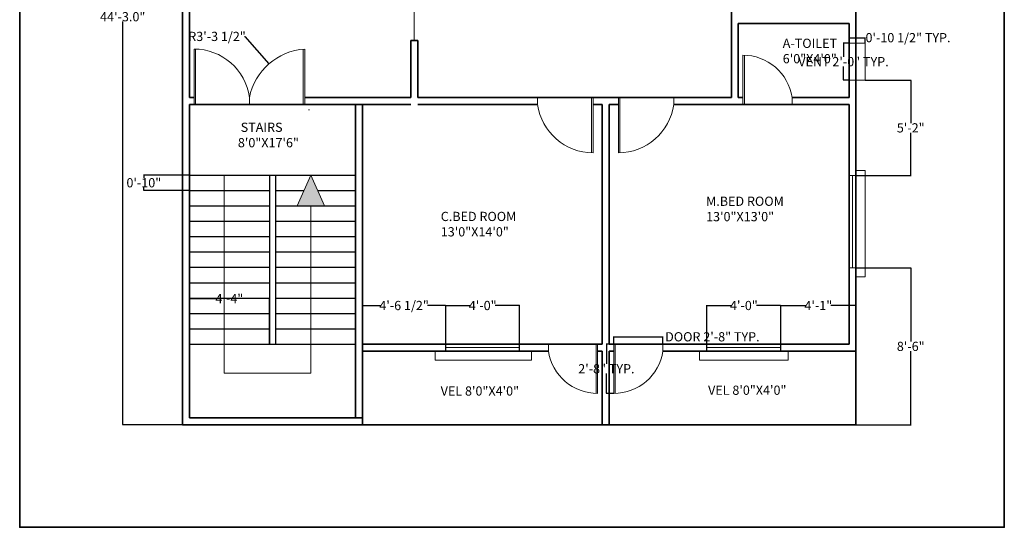
# Model space of a CAD drawing. Units: inches. Extents: x 2946 to 3586, y 7561 to 8235.
# Tile 1 of 2: x 2946 to 3586, y 7561 to 7891. Entities that reach past the tile are written whole.
import ezdxf

# ---------------------------------------------------------------- set-up
doc = ezdxf.new("R2010")
doc.units = ezdxf.units.IN
doc.header["$MEASUREMENT"] = 0
for name, color, linetype, lineweight in [('A-ANNO-DIMS', 2, 'Continuous', 18), ('A-ANNO-PATT', 7, 'Continuous', 18), ('A-ANNO-SYMB', 7, 'Continuous', 18), ('A-ANNO-TTLB', 7, 'Continuous', 35), ('A-AREA-IDEN', 7, 'Continuous', 18), ('A-DOOR', 4, 'Continuous', 18), ('A-FLOR-STRS', 7, 'Continuous', 25), ('A-GLAZ-VENT', 130, 'Continuous', 18), ('A-WALL', 7, 'Continuous', 35), ('windows', 130, 'Continuous', 18)]:
    doc.layers.add(name, color=color, linetype=linetype, lineweight=lineweight)
doc.styles.get("Standard").update_dxf_attribs({"font": 'arial.ttf'})
doc.dimstyles.get("Standard").update_dxf_attribs({"dimtxt": 6, "dimasz": 0.18, "dimexe": 0.18, "dimexo": 0.0625, "dimgap": 0.09, "dimtad": 0, "dimtih": 1, "dimtoh": 1, "dimdec": 1, "dimzin": 0, "dimdsep": 46, "dimlunit": 3, "dimtxsty": 'Standard', "dimcen": 0.09, "dimadec": 0, "dimazin": 0, "dimtfac": 1, "dimtdec": 1, "dimtofl": 0, "dimtmove": 0, "dimatfit": 3, "dimfxl": 1, "dimtolj": 1, "dimtzin": 0, "dimarcsym": 0})

# ---------------------------------------------------------------- blocks, each defined once
blk = doc.blocks.new('*D2')
at = {"layer": 'A-ANNO-DIMS', "color": 0, "lineweight": -2, "transparency": 16777216}
for p, q in [((3051.44, 8158.46), (3012.47, 8158.46)), ((3012.65, 8158.28), (3012.65, 7896.12)), ((3012.65, 7627.64), (3012.65, 7889.81)), ((3051.44, 7627.46), (3012.47, 7627.46))]:
    blk.add_line(p, q, dxfattribs=at)
at = {"layer": 'A-ANNO-DIMS', "color": 0, "transparency": 16777216}
for points in [[(3012.62, 8158.28), (3012.68, 8158.28), (3012.65, 8158.46)], [(3012.62, 7627.64), (3012.68, 7627.64), (3012.65, 7627.46)]]:
    blk.add_solid(points, dxfattribs=at)
at = {"layer": 'Defpoints', "color": 0, "transparency": 16777216}
for p in [(3051.51, 8158.46), (3012.65, 7627.46), (3051.51, 7627.46)]:
    blk.add_point(p, dxfattribs=at)
at = {"layer": 'A-ANNO-DIMS', "color": 0, "transparency": 16777216, "insert": (3012.65, 7892.96), "char_height": 6, "attachment_point": 5}
blk.add_mtext('\\A1;44\'-3.0"', dxfattribs=at)
blk = doc.blocks.new('DOOR-SINGLE-36IN')
for p, q in [((-1, 36), (-1, 0)), ((0, 0), (0, 36)), ((0, 36), (0, 0)), ((-36, 0), (-36, 4.5)), ((0, 0), (-36, 0))]:
    blk.add_line(p, q)
blk.add_arc((0, -0.32), 36.32, 90, 172.37185)
blk = doc.blocks.new('DOOR-SINGLE-32IN')
for p, q in [((0, 0), (0, -32)), ((0, -32), (0, 0)), ((0, 0), (32, 0)), ((1, -32), (1, 0)), ((32, 0), (32, -4.5))]:
    blk.add_line(p, q)
blk.add_arc((0, 0.37), 32.37, 270, 351.34988)
blk = doc.blocks.new('WIN-60IN')
for p, q in [((0, 0), (0, -4.5)), ((60, 0), (0, 0)), ((0, -2.25), (60, -2.25)), ((0, -4.5), (60, -4.5)), ((60, -4.5), (60, 0))]:
    blk.add_line(p, q)
blk = doc.blocks.new('WIN-SILL-60IN')
for p, q in [((0, 0), (0, 6)), ((0, 6), (69.18, 6)), ((69.18, 6), (69.18, 0))]:
    blk.add_line(p, q)
blk = doc.blocks.new('VENT-24IN')
for p, q in [((0, 0), (4.5, 0)), ((0, -24), (0, 0)), ((4.5, 0), (4.5, -24)), ((4.5, 0), (10.5, 0)), ((10.5, 0), (10.5, -24)), ((4.5, -24), (0, -24)), ((10.5, -24), (4.5, -24))]:
    blk.add_line(p, q)
blk = doc.blocks.new('*D14')
at = {"layer": 'A-ANNO-DIMS', "color": 0, "lineweight": -2, "transparency": 16777216}
for p, q in [((3332.01, 7680.02), (3332.01, 7684.94)), ((3332.19, 7684.76), (3363.83, 7684.76)), ((3364.01, 7680.02), (3364.01, 7684.94)), ((3364.01, 7684.76), (3364.19, 7684.76))]:
    blk.add_line(p, q, dxfattribs=at)
at = {"layer": 'A-ANNO-DIMS', "color": 0, "transparency": 16777216}
for points in [[(3332.19, 7684.79), (3332.19, 7684.73), (3332.01, 7684.76)], [(3363.83, 7684.79), (3363.83, 7684.73), (3364.01, 7684.76)]]:
    blk.add_solid(points, dxfattribs=at)
at = {"layer": 'Defpoints', "color": 0, "transparency": 16777216}
for p in [(3364.01, 7684.76), (3332.01, 7679.96), (3364.01, 7679.96)]:
    blk.add_point(p, dxfattribs=at)
at = {"layer": 'A-ANNO-DIMS', "color": 0, "transparency": 16777216, "insert": (3396.15, 7684.76), "char_height": 6, "attachment_point": 5}
blk.add_mtext('\\A1;DOOR 2\'-8" TYP.', dxfattribs=at)
blk = doc.blocks.new('*D15')
at = {"layer": 'A-ANNO-DIMS', "color": 0, "lineweight": -2, "transparency": 16777216}
for p, q in [((3331.94, 7679.96), (3327.03, 7679.96)), ((3327.21, 7679.78), (3327.21, 7667.12)), ((3327.21, 7648.14), (3327.21, 7660.81)), ((3331.94, 7647.96), (3327.03, 7647.96))]:
    blk.add_line(p, q, dxfattribs=at)
at = {"layer": 'A-ANNO-DIMS', "color": 0, "transparency": 16777216}
for points in [[(3327.18, 7679.78), (3327.24, 7679.78), (3327.21, 7679.96)], [(3327.18, 7648.14), (3327.24, 7648.14), (3327.21, 7647.96)]]:
    blk.add_solid(points, dxfattribs=at)
at = {"layer": 'Defpoints', "color": 0, "transparency": 16777216}
for p in [(3327.21, 7679.96), (3332.01, 7679.96), (3332.01, 7647.96)]:
    blk.add_point(p, dxfattribs=at)
at = {"layer": 'A-ANNO-DIMS', "color": 0, "transparency": 16777216, "insert": (3327.21, 7663.96), "char_height": 6, "attachment_point": 5}
blk.add_mtext('\\A1;2\'-8" TYP.', dxfattribs=at)
blk = doc.blocks.new('*D16')
at = {"layer": 'A-ANNO-DIMS', "color": 0, "lineweight": -2, "transparency": 16777216}
for p, q in [((3484.94, 7875.73), (3481.23, 7875.73)), ((3481.41, 7875.55), (3481.41, 7866.89)), ((3481.41, 7851.91), (3481.41, 7860.58)), ((3484.94, 7851.73), (3481.23, 7851.73))]:
    blk.add_line(p, q, dxfattribs=at)
at = {"layer": 'A-ANNO-DIMS', "color": 0, "transparency": 16777216}
for points in [[(3481.38, 7875.55), (3481.44, 7875.55), (3481.41, 7875.73)], [(3481.38, 7851.91), (3481.44, 7851.91), (3481.41, 7851.73)]]:
    blk.add_solid(points, dxfattribs=at)
at = {"layer": 'Defpoints', "color": 0, "transparency": 16777216}
for p in [(3481.41, 7875.73), (3485.01, 7875.73), (3485.01, 7851.73)]:
    blk.add_point(p, dxfattribs=at)
at = {"layer": 'A-ANNO-DIMS', "color": 0, "transparency": 16777216, "insert": (3481.41, 7863.73), "char_height": 6, "attachment_point": 5}
blk.add_mtext('\\A1;VENT 2\'-0" TYP.', dxfattribs=at)
blk = doc.blocks.new('*D17')
at = {"layer": 'A-ANNO-DIMS', "color": 0, "lineweight": -2, "transparency": 16777216}
for p, q in [((3485.01, 7875.79), (3485.01, 7879.51)), ((3485.19, 7879.33), (3495.33, 7879.33)), ((3495.51, 7875.79), (3495.51, 7879.51)), ((3495.51, 7879.33), (3495.69, 7879.33))]:
    blk.add_line(p, q, dxfattribs=at)
at = {"layer": 'A-ANNO-DIMS', "color": 0, "transparency": 16777216}
for points in [[(3485.19, 7879.36), (3485.19, 7879.3), (3485.01, 7879.33)], [(3495.33, 7879.36), (3495.33, 7879.3), (3495.51, 7879.33)]]:
    blk.add_solid(points, dxfattribs=at)
at = {"layer": 'Defpoints', "color": 0, "transparency": 16777216}
for p in [(3495.51, 7879.33), (3485.01, 7875.73), (3495.51, 7875.73)]:
    blk.add_point(p, dxfattribs=at)
at = {"layer": 'A-ANNO-DIMS', "color": 0, "transparency": 16777216, "insert": (3523.39, 7879.33), "char_height": 6, "attachment_point": 5}
blk.add_mtext('\\A1;0\'-10 1/2" TYP.', dxfattribs=at)
blk = doc.blocks.new('*D26')
at = {"layer": 'A-ANNO-DIMS', "color": 0, "lineweight": -2, "transparency": 16777216}
for p, q in [((3495.57, 7851.73), (3525.34, 7851.73)), ((3525.16, 7851.55), (3525.16, 7823.82)), ((3525.16, 7789.79), (3525.16, 7817.52)), ((3489.57, 7789.61), (3525.34, 7789.61))]:
    blk.add_line(p, q, dxfattribs=at)
at = {"layer": 'A-ANNO-DIMS', "color": 0, "transparency": 16777216}
for points in [[(3525.13, 7851.55), (3525.19, 7851.55), (3525.16, 7851.73)], [(3525.13, 7789.79), (3525.19, 7789.79), (3525.16, 7789.61)]]:
    blk.add_solid(points, dxfattribs=at)
at = {"layer": 'Defpoints', "color": 0, "transparency": 16777216}
for p in [(3495.51, 7851.73), (3525.16, 7851.73), (3489.51, 7789.61)]:
    blk.add_point(p, dxfattribs=at)
at = {"layer": 'A-ANNO-DIMS', "color": 0, "transparency": 16777216, "insert": (3525.16, 7820.67), "char_height": 6, "attachment_point": 5}
blk.add_mtext('\\A1;5\'-2"', dxfattribs=at)
blk = doc.blocks.new('*D27')
at = {"layer": 'A-ANNO-DIMS', "color": 0, "lineweight": -2, "transparency": 16777216}
for p, q in [((3489.57, 7729.61), (3525.34, 7729.61)), ((3525.16, 7729.43), (3525.16, 7681.69)), ((3525.16, 7627.64), (3525.16, 7675.38)), ((3489.57, 7627.46), (3525.34, 7627.46))]:
    blk.add_line(p, q, dxfattribs=at)
at = {"layer": 'A-ANNO-DIMS', "color": 0, "transparency": 16777216}
for points in [[(3525.13, 7729.43), (3525.19, 7729.43), (3525.16, 7729.61)], [(3525.13, 7627.64), (3525.19, 7627.64), (3525.16, 7627.46)]]:
    blk.add_solid(points, dxfattribs=at)
at = {"layer": 'Defpoints', "color": 0, "transparency": 16777216}
for p in [(3489.51, 7729.61), (3525.16, 7729.61), (3489.51, 7627.46)]:
    blk.add_point(p, dxfattribs=at)
at = {"layer": 'A-ANNO-DIMS', "color": 0, "transparency": 16777216, "insert": (3525.16, 7678.53), "char_height": 6, "attachment_point": 5}
blk.add_mtext('\\A1;8\'-6"', dxfattribs=at)
blk = doc.blocks.new('*D28')
at = {"layer": 'A-ANNO-DIMS', "color": 0, "lineweight": -2, "transparency": 16777216}
for p, q in [((3056.01, 7680.02), (3056.01, 7709.79)), ((3056.19, 7709.61), (3073.82, 7709.61)), ((3107.83, 7709.61), (3090.19, 7709.61)), ((3108.01, 7680.02), (3108.01, 7709.79))]:
    blk.add_line(p, q, dxfattribs=at)
at = {"layer": 'A-ANNO-DIMS', "color": 0, "transparency": 16777216}
for points in [[(3056.19, 7709.64), (3056.19, 7709.58), (3056.01, 7709.61)], [(3107.83, 7709.64), (3107.83, 7709.58), (3108.01, 7709.61)]]:
    blk.add_solid(points, dxfattribs=at)
at = {"layer": 'Defpoints', "color": 0, "transparency": 16777216}
for p in [(3108.01, 7709.61), (3056.01, 7679.96), (3108.01, 7679.96)]:
    blk.add_point(p, dxfattribs=at)
at = {"layer": 'A-ANNO-DIMS', "color": 0, "transparency": 16777216, "insert": (3082.01, 7709.61), "char_height": 6, "attachment_point": 5}
blk.add_mtext('\\A1;4\'-4"', dxfattribs=at)
blk = doc.blocks.new('*D29')
at = {"layer": 'A-ANNO-DIMS', "color": 0, "lineweight": -2, "transparency": 16777216}
for p, q in [((3055.94, 7789.96), (3026.18, 7789.96)), ((3026.36, 7789.78), (3026.36, 7788.12)), ((3026.36, 7780.14), (3026.36, 7781.81)), ((3055.94, 7779.96), (3026.18, 7779.96))]:
    blk.add_line(p, q, dxfattribs=at)
at = {"layer": 'A-ANNO-DIMS', "color": 0, "transparency": 16777216}
for points in [[(3026.33, 7789.78), (3026.39, 7789.78), (3026.36, 7789.96)], [(3026.33, 7780.14), (3026.39, 7780.14), (3026.36, 7779.96)]]:
    blk.add_solid(points, dxfattribs=at)
at = {"layer": 'Defpoints', "color": 0, "transparency": 16777216}
for p in [(3026.36, 7789.96), (3056.01, 7789.96), (3056.01, 7779.96)]:
    blk.add_point(p, dxfattribs=at)
at = {"layer": 'A-ANNO-DIMS', "color": 0, "transparency": 16777216, "insert": (3026.36, 7784.96), "char_height": 6, "attachment_point": 5}
blk.add_mtext('\\A1;0\'-10"', dxfattribs=at)
blk = doc.blocks.new('*D30')
at = {"layer": 'A-ANNO-DIMS', "color": 0, "lineweight": -2, "transparency": 16777216}
for p, q in [((3168.51, 7675.52), (3168.51, 7705.29)), ((3168.69, 7705.11), (3180.47, 7705.11)), ((3222.6, 7705.11), (3210.82, 7705.11)), ((3222.78, 7675.52), (3222.78, 7705.29))]:
    blk.add_line(p, q, dxfattribs=at)
at = {"layer": 'A-ANNO-DIMS', "color": 0, "transparency": 16777216}
for points in [[(3168.69, 7705.14), (3168.69, 7705.08), (3168.51, 7705.11)], [(3222.6, 7705.14), (3222.6, 7705.08), (3222.78, 7705.11)]]:
    blk.add_solid(points, dxfattribs=at)
at = {"layer": 'Defpoints', "color": 0, "transparency": 16777216}
for p in [(3222.78, 7705.11), (3168.51, 7675.46), (3222.78, 7675.46)]:
    blk.add_point(p, dxfattribs=at)
at = {"layer": 'A-ANNO-DIMS', "color": 0, "transparency": 16777216, "insert": (3195.64, 7705.11), "char_height": 6, "attachment_point": 5}
blk.add_mtext('\\A1;4\'-6 1/2"', dxfattribs=at)
blk = doc.blocks.new('*D31')
at = {"layer": 'A-ANNO-DIMS', "color": 0, "lineweight": -2, "transparency": 16777216}
for p, q in [((3222.78, 7675.52), (3222.78, 7705.29)), ((3222.96, 7705.11), (3238.59, 7705.11)), ((3270.6, 7705.11), (3254.97, 7705.11)), ((3270.78, 7675.52), (3270.78, 7705.29))]:
    blk.add_line(p, q, dxfattribs=at)
at = {"layer": 'A-ANNO-DIMS', "color": 0, "transparency": 16777216}
for points in [[(3222.96, 7705.14), (3222.96, 7705.08), (3222.78, 7705.11)], [(3270.6, 7705.14), (3270.6, 7705.08), (3270.78, 7705.11)]]:
    blk.add_solid(points, dxfattribs=at)
at = {"layer": 'Defpoints', "color": 0, "transparency": 16777216}
for p in [(3270.78, 7705.11), (3222.78, 7675.46), (3270.78, 7675.46)]:
    blk.add_point(p, dxfattribs=at)
at = {"layer": 'A-ANNO-DIMS', "color": 0, "transparency": 16777216, "insert": (3246.78, 7705.11), "char_height": 6, "attachment_point": 5}
blk.add_mtext('\\A1;4\'-0"', dxfattribs=at)
blk = doc.blocks.new('*D32')
at = {"layer": 'A-ANNO-DIMS', "color": 0, "lineweight": -2, "transparency": 16777216}
for p, q in [((3392.63, 7675.52), (3392.63, 7705.29)), ((3392.81, 7705.11), (3408.45, 7705.11)), ((3440.45, 7705.11), (3424.82, 7705.11)), ((3440.63, 7675.52), (3440.63, 7705.29))]:
    blk.add_line(p, q, dxfattribs=at)
at = {"layer": 'A-ANNO-DIMS', "color": 0, "transparency": 16777216}
for points in [[(3392.81, 7705.14), (3392.81, 7705.08), (3392.63, 7705.11)], [(3440.45, 7705.14), (3440.45, 7705.08), (3440.63, 7705.11)]]:
    blk.add_solid(points, dxfattribs=at)
at = {"layer": 'Defpoints', "color": 0, "transparency": 16777216}
for p in [(3440.63, 7705.11), (3392.63, 7675.46), (3440.63, 7675.46)]:
    blk.add_point(p, dxfattribs=at)
at = {"layer": 'A-ANNO-DIMS', "color": 0, "transparency": 16777216, "insert": (3416.63, 7705.11), "char_height": 6, "attachment_point": 5}
blk.add_mtext('\\A1;4\'-0"', dxfattribs=at)
blk = doc.blocks.new('*D33')
at = {"layer": 'A-ANNO-DIMS', "color": 0, "lineweight": -2, "transparency": 16777216}
for p, q in [((3440.63, 7675.52), (3440.63, 7705.29)), ((3440.81, 7705.11), (3456.88, 7705.11)), ((3489.33, 7705.11), (3473.26, 7705.11)), ((3489.51, 7675.52), (3489.51, 7705.29))]:
    blk.add_line(p, q, dxfattribs=at)
at = {"layer": 'A-ANNO-DIMS', "color": 0, "transparency": 16777216}
for points in [[(3440.81, 7705.14), (3440.81, 7705.08), (3440.63, 7705.11)], [(3489.33, 7705.14), (3489.33, 7705.08), (3489.51, 7705.11)]]:
    blk.add_solid(points, dxfattribs=at)
at = {"layer": 'Defpoints', "color": 0, "transparency": 16777216}
for p in [(3489.51, 7705.11), (3440.63, 7675.46), (3489.51, 7675.46)]:
    blk.add_point(p, dxfattribs=at)
at = {"layer": 'A-ANNO-DIMS', "color": 0, "transparency": 16777216, "insert": (3465.07, 7705.11), "char_height": 6, "attachment_point": 5}
blk.add_mtext('\\A1;4\'-1"', dxfattribs=at)
blk = doc.blocks.new('*D34')
at = {"layer": 'A-ANNO-DIMS', "color": 0, "lineweight": -2, "transparency": 16777216}
for p, q in [((3091.88, 7880.15), (3092.06, 7880.15)), ((3092.06, 7880.15), (3107.6, 7862.39)), ((3133.71, 7832.44), (3133.89, 7832.44)), ((3133.8, 7832.35), (3133.8, 7832.53))]:
    blk.add_line(p, q, dxfattribs=at)
at = {"layer": 'A-ANNO-DIMS', "color": 0, "transparency": 16777216}
blk.add_solid([(3107.62, 7862.41), (3107.58, 7862.37), (3107.72, 7862.26)], dxfattribs=at)
at = {"layer": 'Defpoints', "color": 0, "transparency": 16777216}
for p in [(3107.72, 7862.26), (3133.8, 7832.44)]:
    blk.add_point(p, dxfattribs=at)
at = {"layer": 'A-ANNO-DIMS', "color": 0, "transparency": 16777216, "insert": (3073.96, 7880.15), "char_height": 6, "attachment_point": 5}
blk.add_mtext('\\A1;R3\'-3 1/2"', dxfattribs=at)

msp = doc.modelspace()

# ---------------------------------------------------------------- hatches: boundary and pattern name
at = {"layer": 'A-ANNO-PATT'}
h = msp.add_hatch(color=256, dxfattribs=at)
h.dxf.hatch_style = 1
h.paths.add_polyline_path([(3134.98, 7789.96), (3126.01, 7769.96), (3143.96, 7769.96)])

# ---------------------------------------------------------------- linework, layer by layer
at = {"layer": 'A-ANNO-SYMB'}
for p, q in [((3078.69, 7789.96), (3078.69, 7661.05)), ((3134.98, 7789.96), (3126.01, 7769.96)), ((3134.98, 7789.96), (3143.96, 7769.96)), ((3126.01, 7769.96), (3143.96, 7769.96)), ((3134.98, 7661.05), (3134.98, 7769.96)), ((3078.69, 7661.05), (3134.98, 7661.05))]:
    msp.add_line(p, q, dxfattribs=at)
at = {"layer": 'A-ANNO-TTLB'}
msp.add_lwpolyline([(2945.62, 8234.75), (3586.02, 8234.75), (3586.02, 7560.83), (2945.62, 7560.83)], close=True, dxfattribs=at)
at = {"layer": 'A-DOOR'}
for p, q in [((3059.01, 7835.96), (3059.01, 7871.96)), ((3059.01, 7871.96), (3059.01, 7835.96)), ((3060.01, 7871.96), (3060.01, 7835.96)), ((3130.01, 7871.96), (3130.01, 7835.96)), ((3131.01, 7835.96), (3131.01, 7871.96)), ((3131.01, 7871.96), (3131.01, 7835.96)), ((3095.01, 7835.96), (3095.01, 7840.46)), ((3095.01, 7840.46), (3095.01, 7835.96)), ((3059.01, 7835.96), (3095.01, 7835.96)), ((3095.01, 7835.96), (3131.01, 7835.96))]:
    msp.add_line(p, q, dxfattribs=at)
for centre, radius, start, end in [((3059.01, 7835.64), 36.32, 7.62815, 90), ((3133.8, 7832.44), 39.62, 94.04721, 168.32464)]:
    msp.add_arc(centre, radius, start, end, dxfattribs=at)
at = {"layer": 'A-FLOR-STRS'}
for p, q in [((3056.01, 7789.96), (3164.01, 7789.96)), ((3108.01, 7789.96), (3108.01, 7679.96)), ((3112.01, 7789.96), (3112.01, 7679.96)), ((3056.01, 7779.96), (3108.01, 7779.96)), ((3056.01, 7779.96), (3108.01, 7779.96)), ((3112.01, 7779.96), (3130.49, 7779.96)), ((3112.01, 7779.96), (3126.01, 7779.96)), ((3139.47, 7779.96), (3164.01, 7779.96)), ((3056.01, 7769.96), (3108.01, 7769.96)), ((3056.01, 7769.96), (3108.01, 7769.96)), ((3112.01, 7769.96), (3126.01, 7769.96)), ((3112.01, 7769.96), (3164.01, 7769.96)), ((3056.01, 7759.96), (3108.01, 7759.96)), ((3056.01, 7759.96), (3108.01, 7759.96)), ((3112.01, 7759.96), (3126.01, 7759.96)), ((3112.01, 7759.96), (3164.01, 7759.96)), ((3056.01, 7749.96), (3108.01, 7749.96)), ((3056.01, 7749.96), (3108.01, 7749.96)), ((3112.01, 7749.96), (3126.01, 7749.96)), ((3112.01, 7749.96), (3164.01, 7749.96)), ((3056.01, 7739.96), (3108.01, 7739.96)), ((3056.01, 7739.96), (3108.01, 7739.96)), ((3112.01, 7739.96), (3126.01, 7739.96)), ((3112.01, 7739.96), (3164.01, 7739.96)), ((3056.01, 7729.96), (3108.01, 7729.96)), ((3056.01, 7729.96), (3108.01, 7729.96)), ((3112.01, 7729.96), (3164.01, 7729.96)), ((3112.01, 7729.96), (3126.01, 7729.96)), ((3056.01, 7719.96), (3108.01, 7719.96)), ((3056.01, 7719.96), (3108.01, 7719.96)), ((3112.01, 7719.96), (3164.01, 7719.96)), ((3112.01, 7719.96), (3126.01, 7719.96)), ((3056.01, 7709.96), (3108.01, 7709.96)), ((3056.01, 7709.96), (3108.01, 7709.96)), ((3112.01, 7709.96), (3126.01, 7709.96)), ((3112.01, 7709.96), (3164.01, 7709.96)), ((3056.01, 7699.96), (3108.01, 7699.96)), ((3056.01, 7699.96), (3108.01, 7699.96)), ((3112.01, 7699.96), (3126.01, 7699.96)), ((3112.01, 7699.96), (3164.01, 7699.96)), ((3056.01, 7689.96), (3108.01, 7689.96)), ((3056.01, 7689.96), (3108.01, 7689.96)), ((3112.01, 7689.96), (3126.01, 7689.96)), ((3112.01, 7689.96), (3164.01, 7689.96)), ((3056.01, 7679.96), (3164.01, 7679.96))]:
    msp.add_line(p, q, dxfattribs=at)
at = {"layer": 'A-WALL'}
for p, q in [((3051.51, 8158.46), (3051.51, 7627.46)), ((3489.51, 8158.46), (3489.51, 7627.46)), ((3056.01, 7993.46), (3056.01, 7840.46)), ((3408.51, 7993.46), (3408.51, 7840.46)), ((3413.01, 7888.46), (3485.01, 7888.46)), ((3413.01, 7888.46), (3413.01, 7840.46)), ((3485.01, 7888.46), (3485.01, 7840.46)), ((3200.01, 7877.43), (3204.51, 7877.43)), ((3200.01, 7877.43), (3200.01, 7840.46)), ((3204.51, 7877.43), (3204.51, 7840.46)), ((3056.01, 7840.46), (3059.01, 7840.46)), ((3131.01, 7840.46), (3200.01, 7840.46)), ((3204.51, 7840.46), (3408.51, 7840.46)), ((3324.51, 7840.46), (3318.51, 7840.46)), ((3329.01, 7840.46), (3335.01, 7840.46)), ((3413.01, 7840.46), (3416.01, 7840.46)), ((3448.01, 7840.46), (3485.01, 7840.46)), ((3056.01, 7835.96), (3200.01, 7835.96)), ((3056.01, 7835.96), (3059.01, 7835.96)), ((3056.01, 7835.96), (3056.01, 7631.96)), ((3164.01, 7835.96), (3164.01, 7679.96)), ((3168.51, 7835.96), (3168.51, 7679.96)), ((3204.51, 7835.96), (3282.51, 7835.96)), ((3318.51, 7835.96), (3324.51, 7835.96)), ((3324.51, 7835.96), (3324.51, 7679.96)), ((3329.01, 7835.96), (3329.01, 7679.96)), ((3329.01, 7835.96), (3335.01, 7835.96)), ((3371.01, 7835.96), (3485.01, 7835.96)), ((3413.01, 7835.96), (3416.01, 7835.96)), ((3485.01, 7835.96), (3485.01, 7679.96)), ((3164.01, 7679.96), (3164.01, 7631.96)), ((3168.51, 7679.96), (3168.51, 7627.46)), ((3168.51, 7679.96), (3200.01, 7679.96)), ((3200.01, 7679.96), (3324.51, 7679.96)), ((3324.51, 7679.96), (3321.51, 7679.96)), ((3329.01, 7679.96), (3332.01, 7679.96)), ((3329.01, 7679.96), (3485.01, 7679.96)), ((3056.01, 7631.96), (3056.01, 7675.46)), ((3168.51, 7675.46), (3200.01, 7675.46)), ((3200.01, 7675.46), (3289.51, 7675.46)), ((3321.51, 7675.46), (3324.51, 7675.46)), ((3324.51, 7675.46), (3324.51, 7627.46)), ((3329.01, 7675.46), (3329.01, 7627.46)), ((3329.01, 7675.46), (3332.01, 7675.46)), ((3364.01, 7675.46), (3489.51, 7675.46)), ((3051.51, 7631.96), (3051.51, 7631.96)), ((3051.51, 7627.46), (3489.51, 7627.46)), ((3056.01, 7631.96), (3168.51, 7631.96))]:
    msp.add_line(p, q, dxfattribs=at)
at = {"layer": 'windows'}
for p, q in [((3202.26, 7965.14), (3202.26, 7877.43)), ((3222.78, 7679.96), (3222.78, 7675.46)), ((3270.51, 7679.96), (3222.78, 7679.96)), ((3270.78, 7675.46), (3270.51, 7679.96)), ((3392.63, 7675.46), (3392.63, 7679.96)), ((3392.63, 7679.96), (3440.63, 7679.96)), ((3440.63, 7679.96), (3440.63, 7675.46)), ((3215.94, 7669.46), (3215.94, 7675.46)), ((3222.78, 7677.71), (3270.64, 7677.71)), ((3222.78, 7675.46), (3222.78, 7675.46)), ((3222.78, 7675.46), (3270.78, 7675.46)), ((3278.49, 7675.46), (3278.49, 7669.46)), ((3387.86, 7669.46), (3387.86, 7675.46)), ((3392.63, 7677.71), (3440.63, 7677.71)), ((3440.63, 7675.46), (3392.63, 7675.46)), ((3445.4, 7675.46), (3445.4, 7669.46)), ((3278.49, 7669.46), (3215.94, 7669.46)), ((3445.4, 7669.46), (3387.86, 7669.46))]:
    msp.add_line(p, q, dxfattribs=at)

# ---------------------------------------------------------------- block references
at = {"layer": 'A-DOOR', "extrusion": (0, 0, -1), "zscale": -1, "rotation": 180}
for name, p in [('DOOR-SINGLE-32IN', (-3416.01, 7835.96)), ('DOOR-SINGLE-36IN', (-3318.51, 7840.46))]:
    msp.add_blockref(name, p, dxfattribs=at)
at = {"layer": 'A-DOOR', "rotation": 180}
msp.add_blockref('DOOR-SINGLE-36IN', (3335.01, 7840.46), dxfattribs=at)
at = {"layer": 'A-DOOR', "extrusion": (0, 0, -1), "zscale": -1}
msp.add_blockref('DOOR-SINGLE-32IN', (-3321.51, 7679.96), dxfattribs=at)
at = {"layer": 'A-DOOR'}
msp.add_blockref('DOOR-SINGLE-32IN', (3332.01, 7679.96), dxfattribs=at)
at = {"layer": 'A-GLAZ-VENT'}
msp.add_blockref('VENT-24IN', (3485.01, 7875.73), dxfattribs=at)
at = {"layer": 'windows'}
for name, p, rotation in [('WIN-60IN', (3485.01, 7729.61), 90.00000000000202), ('WIN-SILL-60IN', (3489.51, 7793.02), 269.9999999999998)]:
    msp.add_blockref(name, p, dxfattribs=dict(at, rotation=rotation))

# ---------------------------------------------------------------- texts
at = {"layer": 'A-AREA-IDEN', "char_height": 6, "attachment_point": 1}
for s, width, insert in [('A-TOILET\\P6\'0"X4\'0"', 38.2975, (3441.9, 7878.67)), (' STAIRS\\P8\'0"X17\'6"', 71.4212, (3087.53, 7824.04)), ('M.BED ROOM\\P13\'0"X13\'0"', 98.5773, (3392.04, 7775.94)), ('C.BED ROOM\\P13\'0"X14\'0"', 107.1422, (3219.49, 7766.05)), ('VEL 8\'0"X4\'0"', 99.933, (3219.44, 7652.5)), ('VEL 8\'0"X4\'0"', 99.933, (3393.35, 7653.01)), ('VEL 8\'0"X4\'0"', 99.933, (3393.35, 7653.01))]:
    msp.add_mtext_dynamic_manual_height_columns(s, width=width, gutter_width=1, heights=[0], dxfattribs=dict(at, insert=insert))

# ---------------------------------------------------------------- dimensions: what is measured, and where the dimension line sits
at = {"layer": 'A-ANNO-DIMS'}
for base, p1, p2, override, picture, middle in [((3012.65, 7627.46), (3051.51, 8158.46), (3051.51, 7627.46), {"dimclrd": 0, "dimclre": 0, "dimclrt": 0}, '*D2', (3012.65, 7892.96)), ((3525.16, 7851.73), (3489.51, 7789.61), (3495.51, 7851.73), {"dimdec": 1, "dimlfac": 1, "dimrnd": 0, "dimzin": 1, "dimdsep": 46, "dimlunit": 4, "dimfrac": 2}, '*D26', (3525.16, 7820.67)), ((3026.36, 7789.96), (3056.01, 7779.96), (3056.01, 7789.96), {"dimdec": 1, "dimlfac": 1, "dimrnd": 0, "dimzin": 1, "dimdsep": 46, "dimlunit": 4, "dimfrac": 2}, '*D29', (3026.36, 7784.96)), ((3525.1574, 7729.6073), (3489.5074, 7627.4616), (3489.5074, 7729.6073), {"dimdec": 1, "dimlfac": 1, "dimrnd": 0, "dimzin": 1, "dimdsep": 46, "dimlunit": 4, "dimfrac": 2}, '*D27', (3525.1574, 7678.5344))]:
    dim = msp.add_linear_dim(base=base, p1=p1, p2=p2, angle=90, dimstyle='Standard', override=override, dxfattribs=at)
    dim.commit()
    dim.dimension.update_dxf_attribs({"geometry": picture, "text_midpoint": middle})
for base, p1, p2, text, picture, middle in [((3495.51, 7879.33), (3485.01, 7875.73), (3495.51, 7875.73), '<> TYP.', '*D17', (3523.39, 7879.33)), ((3364.01, 7684.76), (3332.01, 7679.96), (3364.01, 7679.96), 'DOOR <> TYP.', '*D14', (3396.15, 7684.76))]:
    dim = msp.add_linear_dim(base=base, p1=p1, p2=p2, text=text, dimstyle='Standard', override={"dimdec": 1, "dimlfac": 1, "dimrnd": 0, "dimzin": 1, "dimdsep": 46, "dimlunit": 4, "dimfrac": 2}, dxfattribs=at)
    dim.commit()
    dim.dimension.update_dxf_attribs({"geometry": picture, "text_midpoint": middle})
dim = msp.add_radius_dim(center=(3133.8, 7832.44), mpoint=(3107.72, 7862.26), dimstyle='Standard', override={"dimdec": 1, "dimlfac": 1, "dimrnd": 0, "dimzin": 1, "dimdsep": 46, "dimlunit": 4, "dimfrac": 2}, dxfattribs=at)
dim.commit()
dim.dimension.update_dxf_attribs({"geometry": '*D34', "text_midpoint": (3073.96, 7880.15), "dimtype": 164})
for base, p1, p2, text, picture, middle in [((3481.41, 7875.73), (3485.01, 7851.73), (3485.01, 7875.73), 'VENT <> TYP.', '*D16', (3481.41, 7863.73)), ((3327.21, 7679.96), (3332.01, 7647.96), (3332.01, 7679.96), '<> TYP.', '*D15', (3327.21, 7663.96))]:
    dim = msp.add_linear_dim(base=base, p1=p1, p2=p2, angle=90, text=text, dimstyle='Standard', override={"dimdec": 1, "dimlfac": 1, "dimrnd": 0, "dimzin": 1, "dimdsep": 46, "dimlunit": 4, "dimfrac": 2}, dxfattribs=at)
    dim.commit()
    dim.dimension.update_dxf_attribs({"geometry": picture, "text_midpoint": middle})
for base, p1, p2, picture, middle in [((3108.01, 7709.61), (3056.01, 7679.96), (3108.01, 7679.96), '*D28', (3082.01, 7709.61)), ((3222.78, 7705.11), (3168.51, 7675.46), (3222.78, 7675.46), '*D30', (3195.64, 7705.11)), ((3270.78, 7705.11), (3222.78, 7675.46), (3270.78, 7675.46), '*D31', (3246.78, 7705.11)), ((3440.63, 7705.11), (3392.63, 7675.46), (3440.63, 7675.46), '*D32', (3416.63, 7705.11)), ((3489.51, 7705.11), (3440.63, 7675.46), (3489.51, 7675.46), '*D33', (3465.07, 7705.11))]:
    dim = msp.add_linear_dim(base=base, p1=p1, p2=p2, dimstyle='Standard', override={"dimdec": 1, "dimlfac": 1, "dimrnd": 0, "dimzin": 1, "dimdsep": 46, "dimlunit": 4, "dimfrac": 2}, dxfattribs=at)
    dim.commit()
    dim.dimension.update_dxf_attribs({"geometry": picture, "text_midpoint": middle})

doc.saveas('drawing.dxf')
